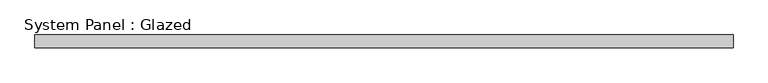
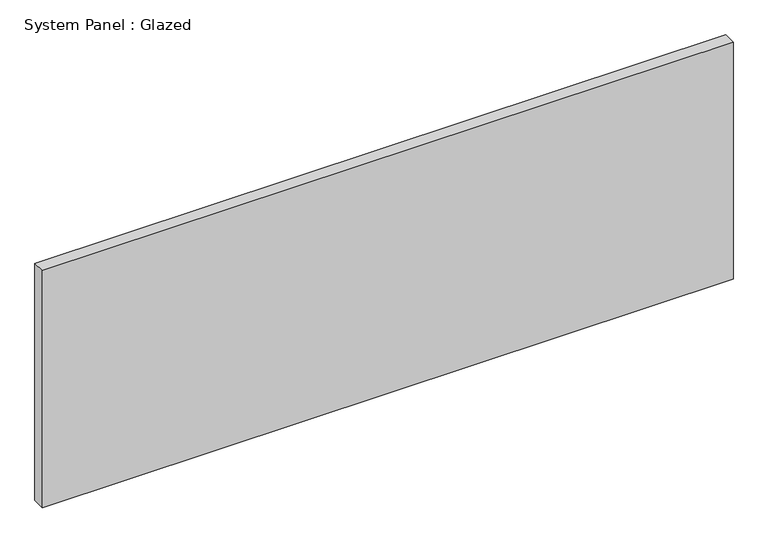
"""IFC4 building model written with IfcOpenShell, lengths in millimetres: plate geometry, System Panel : Glazed."""

from ifc_helpers import new_model, si_unit, origin, origin_with_axes, place, context, project, spatial, polyline, outline, extrude, source, transform, mapped, element, save


def system_panel_glazed_1724a70f(model_context):
    return source(origin(), model_context, "Body", "SweptSolid", [
        extrude(outline(polyline([(688.975, 19.05), (-688.975, 19.05), (-688.975, 44.45), (688.975, 44.45), (688.975, 19.05)])), origin_with_axes(), (0.0, 0.0, 1.0), 500.2736621),
    ])


if __name__ == "__main__":
    model = new_model("IFC4")
    model_context = context("Model", 3, world=origin())
    ifc_project = project(units=[si_unit("LENGTHUNIT", "METRE", prefix="MILLI")], contexts=[model_context])
    site = spatial("IfcSite", under=ifc_project)
    building = spatial("IfcBuilding", under=site)
    placement = place(None, origin())
    system_panel_glazed_shape = system_panel_glazed_1724a70f(model_context)
    element("IfcPlate", 1, ObjectType="System Panel : Glazed", at=placement, inside=building, context=model_context, shape_type="MappedRepresentation", body=[
        mapped(system_panel_glazed_shape, transform((0.0, 0.0, 0.0), x_axis=(1.0, 0.0, 0.0), y_axis=(0.0, 1.0, 0.0), z_axis=(0.0, 0.0, 1.0))),
    ])
    save(model, "model.ifc")

# Revit data of these elements
# Type "System Panel : Glazed"
#   Construction Type Id = "GSP4R"
#   Analytic Construction = "1/8 in Pilkington single glazing"
#   Visual Light Transmittance = 0.9
#   Solar Heat Gain Coefficient = 0.86
#   Heat Transfer Coefficient (U) = 1.18115 BTU/(h·ft²·°F)
#   Define Thermal Properties by = 1
# Element 1 (IfcPlate, "System Panel : Glazed")
#   Materials on its faces: "Glass"
# Materials
#   "Glass": class "Glass", colour RGB 0 128 192, transparency 0.75, Description = "Soda Lime Glass", Cost = 0
